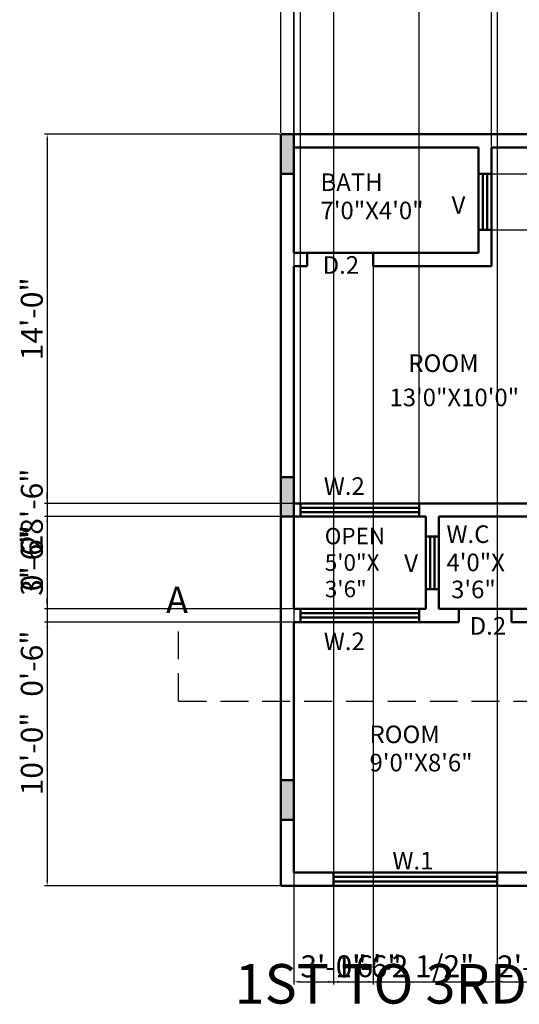
# Model space of a CAD drawing. Units: inches. Extents: x 2368 to 3882, y 1243 to 2139.
# Tile 1 of 6: x 2368 to 2595, y 1243 to 1691. Entities that reach past the tile are written whole.
import ezdxf

# ---------------------------------------------------------------- set-up
doc = ezdxf.new("R2010")
doc.units = ezdxf.units.IN
doc.linetypes.add('DASHED', pattern=[19.05, 12.7, -6.35])
for name, color, linetype, lineweight in [('A-ANNO-DIMS', 2, 'Continuous', 18), ('A-ANNO-SYMB', 1, 'DASHED', 25), ('A-ANNO-TEXT', 7, 'Continuous', 18), ('A-AREA-IDEN', 3, 'Continuous', 18), ('A-WALL', 7, 'Continuous', 50), ('A-WALL-PATT', 8, 'Continuous', 13)]:
    doc.layers.add(name, color=color, linetype=linetype, lineweight=lineweight)
doc.styles.get("Standard").update_dxf_attribs({"font": 'arial.ttf'})
doc.dimstyles.new('ISO-25', dxfattribs={"dimtxt": 10, "dimasz": 2.5, "dimexe": 1.25, "dimexo": 0.625, "dimtad": 1, "dimlunit": 3, "dimtxsty": 'Standard', "dimcen": 2.5, "dimadec": 0, "dimazin": 0, "dimtfac": 1, "dimtmove": 0, "dimatfit": 3, "dimfxl": 1, "dimarcsym": 0})

# ---------------------------------------------------------------- blocks, each defined once
blk = doc.blocks.new('*D33')
at = {"layer": 'A-ANNO-DIMS', "color": 0, "lineweight": -2, "transparency": 16777216}
for p, q in [((2510.5, 1776.18), (2510.5, 1251.93)), ((2492.5, 1770.18), (2492.5, 1251.93)), ((2495, 1253.18), (2508, 1253.18)), ((2510.5, 1253.18), (2539.89, 1253.18))]:
    blk.add_line(p, q, dxfattribs=at)
at = {"layer": 'A-ANNO-DIMS', "color": 0, "transparency": 16777216}
for points in [[(2495, 1253.6), (2495, 1252.77), (2492.5, 1253.18)], [(2508, 1253.6), (2508, 1252.77), (2510.5, 1253.18)]]:
    blk.add_solid(points, dxfattribs=at)
at = {"layer": 'Defpoints', "color": 0, "transparency": 16777216}
for p in [(2510.5, 1776.81), (2492.5, 1770.81), (2510.5, 1253.18)]:
    blk.add_point(p, dxfattribs=at)
at = {"layer": 'A-ANNO-DIMS', "color": 0, "transparency": 16777216, "insert": (2526.44, 1258.91), "char_height": 10, "attachment_point": 5}
blk.add_mtext('1\'-6"', dxfattribs=at)
blk = doc.blocks.new('*D34')
at = {"layer": 'A-ANNO-DIMS', "color": 0, "lineweight": -2, "transparency": 16777216}
for p, q in [((2510.5, 1776.18), (2510.5, 1251.93)), ((2585.04, 1776.18), (2585.04, 1251.93)), ((2513, 1253.18), (2582.54, 1253.18))]:
    blk.add_line(p, q, dxfattribs=at)
at = {"layer": 'A-ANNO-DIMS', "color": 0, "transparency": 16777216}
for points in [[(2513, 1253.6), (2513, 1252.77), (2510.5, 1253.18)], [(2582.54, 1253.6), (2582.54, 1252.77), (2585.04, 1253.18)]]:
    blk.add_solid(points, dxfattribs=at)
at = {"layer": 'Defpoints', "color": 0, "transparency": 16777216}
for p in [(2510.5, 1776.81), (2585.04, 1776.81), (2585.04, 1253.18)]:
    blk.add_point(p, dxfattribs=at)
at = {"layer": 'A-ANNO-DIMS', "color": 0, "transparency": 16777216, "insert": (2547.77, 1258.98), "char_height": 10, "attachment_point": 5}
blk.add_mtext('6\'-2 1/2"', dxfattribs=at)
blk = doc.blocks.new('*D35')
at = {"layer": 'A-ANNO-DIMS', "color": 0, "lineweight": -2, "transparency": 16777216}
for p, q in [((2585.04, 1776.18), (2585.04, 1251.93)), ((2615.04, 1776.18), (2615.04, 1251.93)), ((2587.54, 1253.18), (2612.54, 1253.18))]:
    blk.add_line(p, q, dxfattribs=at)
at = {"layer": 'A-ANNO-DIMS', "color": 0, "transparency": 16777216}
for points in [[(2587.54, 1253.6), (2587.54, 1252.77), (2585.04, 1253.18)], [(2612.54, 1253.6), (2612.54, 1252.77), (2615.04, 1253.18)]]:
    blk.add_solid(points, dxfattribs=at)
at = {"layer": 'Defpoints', "color": 0, "transparency": 16777216}
for p in [(2585.04, 1776.81), (2615.04, 1776.81), (2615.04, 1253.18)]:
    blk.add_point(p, dxfattribs=at)
at = {"layer": 'A-ANNO-DIMS', "color": 0, "transparency": 16777216, "insert": (2600.04, 1258.91), "char_height": 10, "attachment_point": 5}
blk.add_mtext('2\'-6"', dxfattribs=at)
blk = doc.blocks.new('*D38')
at = {"layer": 'A-ANNO-DIMS', "color": 0, "lineweight": -2, "transparency": 16777216}
for p, q in [((2485.87, 1638.88), (2378.96, 1638.88)), ((2380.21, 1636.38), (2380.21, 1299.38)), ((2485.87, 1296.88), (2378.96, 1296.88))]:
    blk.add_line(p, q, dxfattribs=at)
at = {"layer": 'A-ANNO-DIMS', "color": 0, "transparency": 16777216}
for points in [[(2379.79, 1636.38), (2380.63, 1636.38), (2380.21, 1638.88)], [(2379.79, 1299.38), (2380.63, 1299.38), (2380.21, 1296.88)]]:
    blk.add_solid(points, dxfattribs=at)
at = {"layer": 'Defpoints', "color": 0, "transparency": 16777216}
for p in [(2486.5, 1638.88), (2380.21, 1296.88), (2486.5, 1296.88)]:
    blk.add_point(p, dxfattribs=at)
at = {"layer": 'A-ANNO-DIMS', "color": 0, "transparency": 16777216, "insert": (2374.48, 1467.88), "char_height": 10, "attachment_point": 5, "rotation": 90}
blk.add_mtext('28\'-6"', dxfattribs=at)
blk = doc.blocks.new('*D39')
at = {"layer": 'A-ANNO-DIMS', "color": 0, "lineweight": -2, "transparency": 16777216}
for p, q in [((2484, 2126.51), (2481.5, 2126.51)), ((2486.5, 1639.51), (2486.5, 2127.76)), ((2486.5, 2126.51), (2492.5, 2126.51)), ((2492.5, 1633.51), (2492.5, 2127.76)), ((2495, 2126.51), (2525.33, 2126.51))]:
    blk.add_line(p, q, dxfattribs=at)
at = {"layer": 'A-ANNO-DIMS', "color": 0, "transparency": 16777216}
for points in [[(2484, 2126.93), (2484, 2126.09), (2486.5, 2126.51)], [(2495, 2126.93), (2495, 2126.09), (2492.5, 2126.51)]]:
    blk.add_solid(points, dxfattribs=at)
at = {"layer": 'Defpoints', "color": 0, "transparency": 16777216}
for p in [(2492.5, 2126.51), (2486.5, 1638.88), (2492.5, 1632.88)]:
    blk.add_point(p, dxfattribs=at)
at = {"layer": 'A-ANNO-DIMS', "color": 0, "transparency": 16777216, "insert": (2511.41, 2132.24), "char_height": 10, "attachment_point": 5}
blk.add_mtext('0\'-6"', dxfattribs=at)
blk = doc.blocks.new('*D40')
at = {"layer": 'A-ANNO-DIMS', "color": 0, "lineweight": -2, "transparency": 16777216}
for p, q in [((2485.87, 1638.88), (2378.96, 1638.88)), ((2380.21, 1636.38), (2380.21, 1473.38)), ((2491.87, 1470.88), (2378.96, 1470.88))]:
    blk.add_line(p, q, dxfattribs=at)
at = {"layer": 'A-ANNO-DIMS', "color": 0, "transparency": 16777216}
for points in [[(2379.79, 1636.38), (2380.63, 1636.38), (2380.21, 1638.88)], [(2379.79, 1473.38), (2380.63, 1473.38), (2380.21, 1470.88)]]:
    blk.add_solid(points, dxfattribs=at)
at = {"layer": 'Defpoints', "color": 0, "transparency": 16777216}
for p in [(2486.5, 1638.88), (2380.21, 1470.88), (2492.5, 1470.88)]:
    blk.add_point(p, dxfattribs=at)
at = {"layer": 'A-ANNO-DIMS', "color": 0, "transparency": 16777216, "insert": (2374.48, 1554.88), "char_height": 10, "attachment_point": 5, "rotation": 90}
blk.add_mtext('14\'-0"', dxfattribs=at)
blk = doc.blocks.new('*D41')
at = {"layer": 'A-ANNO-DIMS', "color": 0, "lineweight": -2, "transparency": 16777216}
for p, q in [((2380.21, 1473.38), (2380.21, 1475.88)), ((2491.87, 1470.88), (2378.96, 1470.88)), ((2380.21, 1470.88), (2380.21, 1464.88)), ((2491.87, 1464.88), (2378.96, 1464.88)), ((2380.21, 1462.38), (2380.21, 1432.05))]:
    blk.add_line(p, q, dxfattribs=at)
at = {"layer": 'A-ANNO-DIMS', "color": 0, "transparency": 16777216}
for points in [[(2379.79, 1473.38), (2380.63, 1473.38), (2380.21, 1470.88)], [(2379.79, 1462.38), (2380.63, 1462.38), (2380.21, 1464.88)]]:
    blk.add_solid(points, dxfattribs=at)
at = {"layer": 'Defpoints', "color": 0, "transparency": 16777216}
for p in [(2492.5, 1470.88), (2380.21, 1464.88), (2492.5, 1464.88)]:
    blk.add_point(p, dxfattribs=at)
at = {"layer": 'A-ANNO-DIMS', "color": 0, "transparency": 16777216, "insert": (2374.48, 1445.97), "char_height": 10, "attachment_point": 5, "rotation": 90}
blk.add_mtext('0\'-6"', dxfattribs=at)
blk = doc.blocks.new('*D42')
at = {"layer": 'A-ANNO-DIMS', "color": 0, "lineweight": -2, "transparency": 16777216}
for p, q in [((2491.87, 1464.88), (2378.96, 1464.88)), ((2380.21, 1462.38), (2380.21, 1425.38)), ((2491.87, 1422.88), (2378.96, 1422.88))]:
    blk.add_line(p, q, dxfattribs=at)
at = {"layer": 'A-ANNO-DIMS', "color": 0, "transparency": 16777216}
for points in [[(2379.79, 1462.38), (2380.63, 1462.38), (2380.21, 1464.88)], [(2379.79, 1425.38), (2380.63, 1425.38), (2380.21, 1422.88)]]:
    blk.add_solid(points, dxfattribs=at)
at = {"layer": 'Defpoints', "color": 0, "transparency": 16777216}
for p in [(2492.5, 1464.88), (2380.21, 1422.88), (2492.5, 1422.88)]:
    blk.add_point(p, dxfattribs=at)
at = {"layer": 'A-ANNO-DIMS', "color": 0, "transparency": 16777216, "insert": (2374.48, 1443.88), "char_height": 10, "attachment_point": 5, "rotation": 90}
blk.add_mtext('3\'-6"', dxfattribs=at)
blk = doc.blocks.new('*D43')
at = {"layer": 'A-ANNO-DIMS', "color": 0, "lineweight": -2, "transparency": 16777216}
for p, q in [((2380.21, 1425.38), (2380.21, 1427.88)), ((2491.87, 1422.88), (2378.96, 1422.88)), ((2380.21, 1422.88), (2380.21, 1416.88)), ((2491.87, 1416.88), (2378.96, 1416.88)), ((2380.21, 1414.38), (2380.21, 1384.05))]:
    blk.add_line(p, q, dxfattribs=at)
at = {"layer": 'A-ANNO-DIMS', "color": 0, "transparency": 16777216}
for points in [[(2379.79, 1425.38), (2380.63, 1425.38), (2380.21, 1422.88)], [(2379.79, 1414.38), (2380.63, 1414.38), (2380.21, 1416.88)]]:
    blk.add_solid(points, dxfattribs=at)
at = {"layer": 'Defpoints', "color": 0, "transparency": 16777216}
for p in [(2492.5, 1422.88), (2380.21, 1416.88), (2492.5, 1416.88)]:
    blk.add_point(p, dxfattribs=at)
at = {"layer": 'A-ANNO-DIMS', "color": 0, "transparency": 16777216, "insert": (2374.48, 1397.97), "char_height": 10, "attachment_point": 5, "rotation": 90}
blk.add_mtext('0\'-6"', dxfattribs=at)
blk = doc.blocks.new('*D44')
at = {"layer": 'A-ANNO-DIMS', "color": 0, "lineweight": -2, "transparency": 16777216}
for p, q in [((2491.87, 1416.88), (2378.96, 1416.88)), ((2380.21, 1414.38), (2380.21, 1299.38)), ((2485.87, 1296.88), (2378.96, 1296.88))]:
    blk.add_line(p, q, dxfattribs=at)
at = {"layer": 'A-ANNO-DIMS', "color": 0, "transparency": 16777216}
for points in [[(2379.79, 1414.38), (2380.63, 1414.38), (2380.21, 1416.88)], [(2379.79, 1299.38), (2380.63, 1299.38), (2380.21, 1296.88)]]:
    blk.add_solid(points, dxfattribs=at)
at = {"layer": 'Defpoints', "color": 0, "transparency": 16777216}
for p in [(2492.5, 1416.88), (2380.21, 1296.88), (2486.5, 1296.88)]:
    blk.add_point(p, dxfattribs=at)
at = {"layer": 'A-ANNO-DIMS', "color": 0, "transparency": 16777216, "insert": (2374.48, 1356.88), "char_height": 10, "attachment_point": 5, "rotation": 90}
blk.add_mtext('10\'-0"', dxfattribs=at)
blk = doc.blocks.new('*D50')
at = {"layer": 'A-ANNO-DIMS', "color": 0, "lineweight": -2, "transparency": 16777216}
for p, q in [((2582.5, 1633.51), (2582.5, 2127.76)), ((2585, 2126.51), (2646, 2126.51)), ((2648.5, 1639.51), (2648.5, 2127.76))]:
    blk.add_line(p, q, dxfattribs=at)
at = {"layer": 'A-ANNO-DIMS', "color": 0, "transparency": 16777216}
for points in [[(2585, 2126.93), (2585, 2126.09), (2582.5, 2126.51)], [(2646, 2126.93), (2646, 2126.09), (2648.5, 2126.51)]]:
    blk.add_solid(points, dxfattribs=at)
at = {"layer": 'Defpoints', "color": 0, "transparency": 16777216}
for p in [(2648.5, 2126.51), (2648.5, 1638.88), (2582.5, 1632.88)]:
    blk.add_point(p, dxfattribs=at)
at = {"layer": 'A-ANNO-DIMS', "color": 0, "transparency": 16777216, "insert": (2615.5, 2132.24), "char_height": 10, "attachment_point": 5}
blk.add_mtext('5\'-6"', dxfattribs=at)
blk = doc.blocks.new('*D52')
at = {"layer": 'A-ANNO-DIMS', "color": 0, "lineweight": -2, "transparency": 16777216}
for p, q in [((2492.5, 1633.51), (2492.5, 2127.76)), ((2495, 2126.51), (2580, 2126.51)), ((2582.5, 1633.51), (2582.5, 2127.76))]:
    blk.add_line(p, q, dxfattribs=at)
at = {"layer": 'A-ANNO-DIMS', "color": 0, "transparency": 16777216}
for points in [[(2495, 2126.93), (2495, 2126.09), (2492.5, 2126.51)], [(2580, 2126.93), (2580, 2126.09), (2582.5, 2126.51)]]:
    blk.add_solid(points, dxfattribs=at)
at = {"layer": 'Defpoints', "color": 0, "transparency": 16777216}
for p in [(2582.5, 2126.51), (2492.5, 1632.88), (2582.5, 1632.88)]:
    blk.add_point(p, dxfattribs=at)
at = {"layer": 'A-ANNO-DIMS', "color": 0, "transparency": 16777216, "insert": (2537.5, 2132.24), "char_height": 10, "attachment_point": 5}
blk.add_mtext('7\'-6"', dxfattribs=at)
blk = doc.blocks.new('*D54')
at = {"layer": 'A-ANNO-DIMS', "color": 0, "lineweight": -2, "transparency": 16777216}
for p, q in [((2510.5, 1296.26), (2510.5, 1251.93)), ((2585.04, 1296.26), (2585.04, 1251.93)), ((2513, 1253.18), (2582.54, 1253.18))]:
    blk.add_line(p, q, dxfattribs=at)
at = {"layer": 'A-ANNO-DIMS', "color": 0, "transparency": 16777216}
for points in [[(2513, 1253.6), (2513, 1252.77), (2510.5, 1253.18)], [(2582.54, 1253.6), (2582.54, 1252.77), (2585.04, 1253.18)]]:
    blk.add_solid(points, dxfattribs=at)
at = {"layer": 'Defpoints', "color": 0, "transparency": 16777216}
for p in [(2510.5, 1296.88), (2585.04, 1296.88), (2585.04, 1253.18)]:
    blk.add_point(p, dxfattribs=at)
at = {"layer": 'A-ANNO-DIMS', "color": 0, "transparency": 16777216, "insert": (2547.77, 1258.98), "char_height": 10, "attachment_point": 5}
blk.add_mtext('6\'-2 1/2"', dxfattribs=at)
blk = doc.blocks.new('*D55')
at = {"layer": 'A-ANNO-DIMS', "color": 0, "lineweight": -2, "transparency": 16777216}
for p, q in [((2585.04, 1296.26), (2585.04, 1251.93)), ((2606.5, 1296.26), (2606.5, 1251.93)), ((2587.54, 1253.18), (2604, 1253.18)), ((2606.5, 1253.18), (2659.19, 1253.18))]:
    blk.add_line(p, q, dxfattribs=at)
at = {"layer": 'A-ANNO-DIMS', "color": 0, "transparency": 16777216}
for points in [[(2587.54, 1253.6), (2587.54, 1252.77), (2585.04, 1253.18)], [(2604, 1253.6), (2604, 1252.77), (2606.5, 1253.18)]]:
    blk.add_solid(points, dxfattribs=at)
at = {"layer": 'Defpoints', "color": 0, "transparency": 16777216}
for p in [(2585.04, 1296.88), (2606.5, 1296.88), (2606.5, 1253.18)]:
    blk.add_point(p, dxfattribs=at)
at = {"layer": 'A-ANNO-DIMS', "color": 0, "transparency": 16777216, "insert": (2634.09, 1258.98), "char_height": 10, "attachment_point": 5}
blk.add_mtext('1\'-9 1/2"', dxfattribs=at)
blk = doc.blocks.new('*D58')
at = {"layer": 'A-ANNO-DIMS', "color": 0, "lineweight": -2, "transparency": 16777216}
for p, q in [((2495.5, 1471.51), (2495.5, 2127.76)), ((2498, 2126.51), (2547, 2126.51)), ((2549.5, 1471.51), (2549.5, 2127.76))]:
    blk.add_line(p, q, dxfattribs=at)
at = {"layer": 'A-ANNO-DIMS', "color": 0, "transparency": 16777216}
for points in [[(2498, 2126.93), (2498, 2126.09), (2495.5, 2126.51)], [(2547, 2126.93), (2547, 2126.09), (2549.5, 2126.51)]]:
    blk.add_solid(points, dxfattribs=at)
at = {"layer": 'Defpoints', "color": 0, "transparency": 16777216}
for p in [(2549.5, 2126.51), (2495.5, 1470.88), (2549.5, 1470.88)]:
    blk.add_point(p, dxfattribs=at)
at = {"layer": 'A-ANNO-DIMS', "color": 0, "transparency": 16777216, "insert": (2522.5, 2132.24), "char_height": 10, "attachment_point": 5}
blk.add_mtext('4\'-6"', dxfattribs=at)
blk = doc.blocks.new('*D62')
at = {"layer": 'A-ANNO-DIMS', "color": 0, "lineweight": -2, "transparency": 16777216}
for p, q in [((2492.5, 1584.26), (2492.5, 1251.93)), ((2528.5, 1584.26), (2528.5, 1251.93)), ((2495, 1253.18), (2526, 1253.18))]:
    blk.add_line(p, q, dxfattribs=at)
at = {"layer": 'A-ANNO-DIMS', "color": 0, "transparency": 16777216}
for points in [[(2495, 1253.6), (2495, 1252.77), (2492.5, 1253.18)], [(2526, 1253.6), (2526, 1252.77), (2528.5, 1253.18)]]:
    blk.add_solid(points, dxfattribs=at)
at = {"layer": 'Defpoints', "color": 0, "transparency": 16777216}
for p in [(2492.5, 1584.88), (2528.5, 1584.88), (2528.5, 1253.18)]:
    blk.add_point(p, dxfattribs=at)
at = {"layer": 'A-ANNO-DIMS', "color": 0, "transparency": 16777216, "insert": (2510.5, 1258.92), "char_height": 10, "attachment_point": 5}
blk.add_mtext('3\'-0"', dxfattribs=at)
blk = doc.blocks.new('*D63')
at = {"layer": 'A-ANNO-DIMS', "color": 0, "lineweight": -2, "transparency": 16777216}
for p, q in [((2577.12, 1620.88), (2851.45, 1620.88)), ((2850.2, 1618.38), (2850.2, 1597.8)), ((2577.12, 1595.3), (2851.45, 1595.3)), ((2850.2, 1595.3), (2850.2, 1541.5))]:
    blk.add_line(p, q, dxfattribs=at)
at = {"layer": 'A-ANNO-DIMS', "color": 0, "transparency": 16777216}
for points in [[(2849.79, 1618.38), (2850.62, 1618.38), (2850.2, 1620.88)], [(2849.79, 1597.8), (2850.62, 1597.8), (2850.2, 1595.3)]]:
    blk.add_solid(points, dxfattribs=at)
at = {"layer": 'Defpoints', "color": 0, "transparency": 16777216}
for p in [(2576.5, 1620.88), (2576.5, 1595.3), (2850.2, 1595.3)]:
    blk.add_point(p, dxfattribs=at)
at = {"layer": 'A-ANNO-DIMS', "color": 0, "transparency": 16777216, "insert": (2844.41, 1567.15), "char_height": 10, "attachment_point": 5, "rotation": 90}
blk.add_mtext('2\'-1 1/2"', dxfattribs=at)

msp = doc.modelspace()

# ---------------------------------------------------------------- hatches: boundary and pattern name
at = {"layer": 'A-WALL-PATT'}
h = msp.add_hatch(color=256, dxfattribs=at)
h.dxf.hatch_style = 1
h.paths.add_polyline_path([(2492.497, 1344.883), (2486.497, 1344.883), (2486.497, 1326.883), (2492.497, 1326.883)])
h.paths.add_polyline_path([(2618.497, 1332.883), (2600.497, 1332.883), (2600.497, 1326.883), (2618.497, 1326.883)])
h.paths.add_polyline_path([(2744.497, 1344.883), (2738.497, 1344.883), (2738.497, 1326.883), (2744.497, 1326.883)])
h.paths.add_polyline_path([(2744.497, 1482.883), (2738.497, 1482.883), (2738.497, 1464.883), (2744.497, 1464.883)])
h.paths.add_polyline_path([(2660.497, 1470.883), (2642.497, 1470.883), (2642.497, 1464.883), (2660.497, 1464.883)])
h.paths.add_polyline_path([(2492.497, 1482.883), (2486.497, 1482.883), (2486.497, 1464.883), (2492.497, 1464.883)])
h.paths.add_polyline_path([(2492.497, 1638.883), (2486.497, 1638.883), (2486.497, 1620.883), (2492.497, 1620.883)])
h.paths.add_polyline_path([(2654.497, 1638.883), (2648.497, 1638.883), (2648.497, 1620.883), (2654.497, 1620.883)])
h.paths.add_polyline_path([(2744.497, 1638.883), (2738.497, 1638.883), (2738.497, 1620.883), (2744.497, 1620.883)])
h.paths.add_polyline_path([(2744.497, 1788.809), (2738.497, 1788.809), (2738.497, 1770.809), (2744.497, 1770.809)])
h.paths.add_polyline_path([(2615.041, 1776.809), (2597.041, 1776.809), (2597.041, 1770.809), (2615.041, 1770.809)])
h.paths.add_polyline_path([(2492.497, 1788.809), (2486.497, 1788.809), (2486.497, 1770.809), (2492.497, 1770.809)])
h.paths.add_polyline_path([(2492.497, 1926.809), (2486.497, 1926.809), (2486.497, 1908.809), (2492.497, 1908.809)])
h.paths.add_polyline_path([(2660.497, 1914.809), (2642.497, 1914.809), (2642.497, 1908.809), (2660.497, 1908.809)])
h.paths.add_polyline_path([(2744.497, 1926.809), (2738.497, 1926.809), (2738.497, 1908.809), (2744.497, 1908.809)])
h.paths.add_polyline_path([(2744.497, 2082.809), (2738.497, 2082.809), (2738.497, 2064.809), (2744.497, 2064.809)])
h.paths.add_polyline_path([(2654.497, 2082.809), (2648.497, 2082.809), (2648.497, 2064.809), (2654.497, 2064.809)])
h.paths.add_polyline_path([(2492.497, 2082.809), (2486.497, 2082.809), (2486.497, 2064.809), (2492.497, 2064.809)])

# ---------------------------------------------------------------- linework, layer by layer
at = {"layer": 'A-ANNO-SYMB'}
for q in [(2440.007, 1417.69), (2806.503, 1380.883)]:
    msp.add_line((2440.007, 1380.883), q, dxfattribs=at)
at = {"layer": 'A-WALL'}
for p, q in [((2744.497, 1638.883), (2486.497, 1638.883)), ((2486.497, 1638.883), (2486.497, 1296.883)), ((2492.497, 1638.883), (2492.497, 1584.883)), ((2576.497, 1632.883), (2492.497, 1632.883)), ((2576.497, 1632.883), (2576.497, 1584.883)), ((2648.497, 1632.883), (2582.497, 1632.883)), ((2582.497, 1632.883), (2582.497, 1578.883)), ((2492.497, 1620.883), (2486.497, 1620.883)), ((2582.497, 1620.883), (2576.497, 1620.883)), ((2578.497, 1620.883), (2578.497, 1595.303)), ((2580.497, 1620.883), (2580.497, 1595.303)), ((2582.497, 1595.303), (2576.497, 1595.303)), ((2576.497, 1584.883), (2492.497, 1584.883)), ((2498.497, 1584.883), (2498.497, 1578.883)), ((2528.497, 1584.883), (2528.497, 1578.883)), ((2492.497, 1578.883), (2492.497, 1422.883)), ((2498.497, 1578.883), (2492.497, 1578.883)), ((2582.497, 1578.883), (2528.497, 1578.883)), ((2492.497, 1482.883), (2486.497, 1482.883)), ((2492.497, 1470.883), (2606.497, 1470.883)), ((2495.497, 1470.883), (2495.497, 1464.883)), ((2549.497, 1470.883), (2549.497, 1464.883)), ((2495.497, 1468.883), (2549.497, 1468.883)), ((2549.497, 1466.883), (2495.497, 1466.883)), ((2492.497, 1464.883), (2486.497, 1464.883)), ((2492.497, 1464.883), (2552.497, 1464.883)), ((2552.497, 1464.883), (2552.497, 1422.883)), ((2558.497, 1464.883), (2558.497, 1422.883)), ((2558.497, 1464.883), (2600.497, 1464.883)), ((2552.497, 1455.883), (2558.497, 1455.883)), ((2554.497, 1431.883), (2554.497, 1455.883)), ((2556.497, 1455.883), (2556.497, 1431.883)), ((2552.497, 1431.883), (2558.497, 1431.883)), ((2492.497, 1422.883), (2552.497, 1422.883)), ((2495.497, 1422.883), (2495.497, 1416.883)), ((2495.497, 1420.883), (2549.497, 1420.883)), ((2549.497, 1422.883), (2549.497, 1416.883)), ((2558.497, 1422.883), (2600.497, 1422.883)), ((2567.497, 1422.883), (2567.497, 1416.883)), ((2591.497, 1422.883), (2591.497, 1416.883)), ((2492.497, 1416.883), (2567.497, 1416.883)), ((2492.497, 1416.883), (2492.497, 1302.883)), ((2549.497, 1418.883), (2495.497, 1418.883)), ((2591.497, 1416.883), (2606.497, 1416.883)), ((2492.497, 1344.883), (2486.497, 1344.883)), ((2492.497, 1326.883), (2486.497, 1326.883)), ((2492.497, 1302.883), (2600.497, 1302.883)), ((2510.497, 1302.883), (2510.497, 1296.883)), ((2510.497, 1300.883), (2585.041, 1300.883)), ((2585.041, 1302.883), (2585.041, 1296.883)), ((2486.497, 1296.883), (2744.497, 1296.883)), ((2510.497, 1298.883), (2585.041, 1298.883))]:
    msp.add_line(p, q, dxfattribs=at)

# ---------------------------------------------------------------- texts
at = {"layer": 'A-ANNO-SYMB'}
msp.add_text('A', height=12, dxfattribs=at).set_placement((2434.307, 1420.988))
at = {"layer": 'A-ANNO-TEXT'}
for s, height, p in [('V', 8, (2564.26, 1602.684)), ('D.2', 8, (2505.558, 1575.37)), ('W.2', 8, (2506.081, 1474.761)), ('V', 8, (2542.704, 1439.649)), ('D.2', 8, (2572.495, 1411.135)), ('W.2', 8, (2506.081, 1404.1)), ('W.1', 8, (2537.323, 1304.292)), ('1ST TO 3RD FLOOR PLAN', 18, (2465.517, 1243.248))]:
    msp.add_text(s, height=height, dxfattribs=at).set_placement(p)
at = {"layer": 'A-AREA-IDEN'}
for s, p in [('BATH ', (2504.586, 1613.032)), ('7\'0"X4\'0"', (2504.586, 1600.18)), ('ROOM', (2544.566, 1530.682)), ('13\'0"X10\'0"', (2535.964, 1515.097)), ('W.C', (2561.922, 1452.868)), ('4\'0"X', (2561.922, 1440.016)), ('3\'6"', (2564.031, 1427.725)), ('ROOM', (2526.903, 1361.771)), ('9\'0"X8\'6"', (2526.903, 1348.92))]:
    msp.add_text(s, height=8, dxfattribs=at).set_placement(p)
for s, p in [('OPEN', (2506.521, 1452.226)), ('5\'0"X', (2506.556, 1440.188)), ('3\'6"', (2506.591, 1428.149))]:
    msp.add_text(s, height=7.4943, rotation=0.16667, dxfattribs=at).set_placement(p)

# ---------------------------------------------------------------- dimensions: what is measured, and where the dimension line sits
at = {"layer": 'A-ANNO-DIMS'}
for base, p1, p2, picture, middle in [((2492.497, 2126.509), (2486.497, 1638.883), (2492.497, 1632.883), '*D39', (2511.414, 2132.24)), ((2582.497, 2126.509), (2492.497, 1632.883), (2582.497, 1632.883), '*D52', (2537.497, 2132.24)), ((2549.497, 2126.509), (2495.497, 1470.883), (2549.497, 1470.883), '*D58', (2522.497, 2132.24)), ((2648.497, 2126.509), (2582.497, 1632.883), (2648.497, 1638.883), '*D50', (2615.497, 2132.24)), ((2510.497, 1253.183), (2492.497, 1770.809), (2510.497, 1776.809), '*D33', (2526.443, 1258.914)), ((2585.041, 1253.183), (2510.497, 1776.809), (2585.041, 1776.809), '*D34', (2547.769, 1258.979)), ((2615.041, 1253.183), (2585.041, 1776.809), (2615.041, 1776.809), '*D35', (2600.041, 1258.914)), ((2528.497, 1253.183), (2492.497, 1584.883), (2528.497, 1584.883), '*D62', (2510.497, 1258.917)), ((2585.041, 1253.183), (2510.497, 1296.883), (2585.041, 1296.883), '*D54', (2547.769, 1258.979)), ((2606.497, 1253.183), (2585.041, 1296.883), (2606.497, 1296.883), '*D55', (2634.094, 1258.979))]:
    dim = msp.add_linear_dim(base=base, p1=p1, p2=p2, dimstyle='ISO-25', override={"dimdec": 1, "dimlfac": 1, "dimrnd": 0, "dimzin": 1, "dimdsep": 46, "dimlunit": 4, "dimfrac": 2}, dxfattribs=at)
    dim.commit()
    dim.dimension.update_dxf_attribs({"geometry": picture, "text_midpoint": middle})
for base, p1, p2, picture, middle in [((2380.21, 1296.883), (2486.497, 1638.883), (2486.497, 1296.883), '*D38', (2374.48, 1467.883)), ((2380.21, 1470.883), (2486.497, 1638.883), (2492.497, 1470.883), '*D40', (2374.48, 1554.883)), ((2850.203, 1595.303), (2576.497, 1620.883), (2576.497, 1595.303), '*D63', (2844.408, 1567.15)), ((2380.21, 1464.883), (2492.497, 1470.883), (2492.497, 1464.883), '*D41', (2374.48, 1445.967)), ((2380.21, 1422.883), (2492.497, 1464.883), (2492.497, 1422.883), '*D42', (2374.476, 1443.883)), ((2380.21, 1416.883), (2492.497, 1422.883), (2492.497, 1416.883), '*D43', (2374.48, 1397.967)), ((2380.21, 1296.883), (2492.497, 1416.883), (2486.497, 1296.883), '*D44', (2374.48, 1356.883))]:
    dim = msp.add_linear_dim(base=base, p1=p1, p2=p2, angle=90, dimstyle='ISO-25', override={"dimdec": 1, "dimlfac": 1, "dimrnd": 0, "dimzin": 1, "dimdsep": 46, "dimlunit": 4, "dimfrac": 2}, dxfattribs=at)
    dim.commit()
    dim.dimension.update_dxf_attribs({"geometry": picture, "text_midpoint": middle})

doc.saveas('drawing.dxf')
